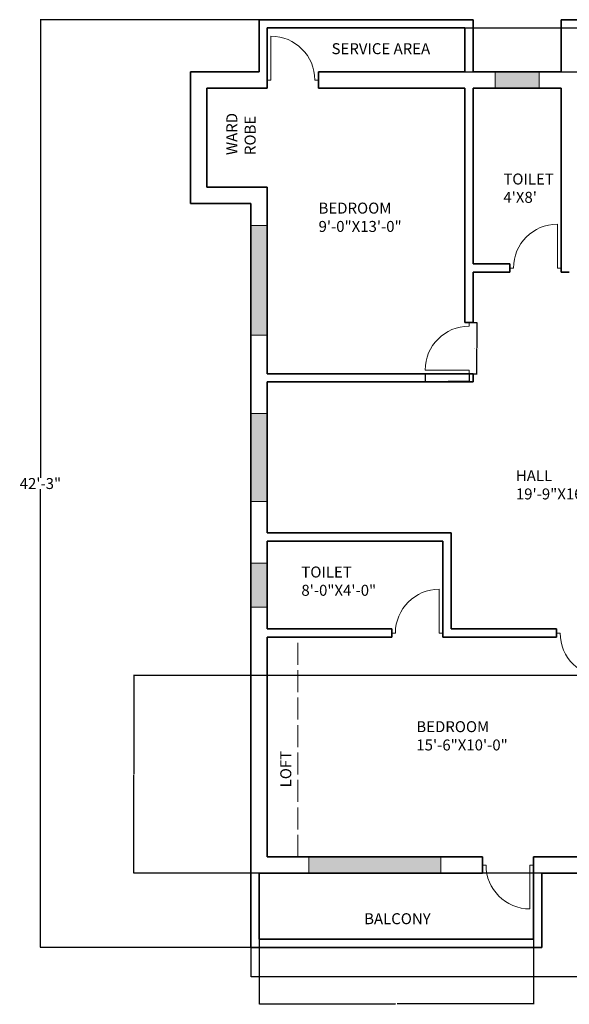
# Model space of a CAD drawing. Units: inches. Extents: x -89 to 565, y -517 to 71.
# Tile 1 of 3: x -89 to 211, y -499 to 39. Entities that reach past the tile are written whole.
import ezdxf

# ---------------------------------------------------------------- set-up
doc = ezdxf.new("R2010")
doc.units = ezdxf.units.IN
doc.header["$MEASUREMENT"] = 0
doc.linetypes.add('ACAD_ISO02W100', pattern=[15, 12, -3])
for name, color, linetype, lineweight in [('A-ANNO-DIMS', 2, 'Continuous', 18), ('A-AREA-IDEN', 7, 'Continuous', 18), ('A-DOOR', 4, 'Continuous', 18), ('A-FLOR-OVHD', 8, 'ACAD_ISO02W100', 18), ('A-GLAZ', 3, 'Continuous', 18), ('A-GLAZ-PATT', 9, 'Continuous', 13), ('A-WALL', 7, 'Continuous', 35)]:
    doc.layers.add(name, color=color, linetype=linetype, lineweight=lineweight)
doc.styles.get("Standard").update_dxf_attribs({"font": 'arial.ttf'})
doc.dimstyles.get("Standard").update_dxf_attribs({"dimtxt": 0.18, "dimasz": 0.18, "dimexe": 0.18, "dimexo": 0.0625, "dimgap": 0.09, "dimtad": 0, "dimtih": 1, "dimtoh": 1, "dimdec": 0, "dimzin": 0, "dimdsep": 46, "dimlunit": 3, "dimtxsty": 'Standard', "dimcen": 0.09, "dimadec": 0, "dimazin": 0, "dimtfac": 1, "dimtdec": 0, "dimtofl": 0, "dimtmove": 0, "dimatfit": 3, "dimfxl": 1, "dimtolj": 1, "dimtzin": 0, "dimarcsym": 0})

# ---------------------------------------------------------------- blocks, each defined once
blk = doc.blocks.new('*D2')
at = {"layer": 'A-ANNO-DIMS', "color": 0, "lineweight": -2, "transparency": 16777216}
for p, q in [((37.09, -467.65), (37.09, -483.62)), ((533.59, -467.65), (533.59, -483.62)), ((37.27, -483.44), (274.83, -483.44)), ((533.41, -483.44), (295.86, -483.44))]:
    blk.add_line(p, q, dxfattribs=at)
at = {"layer": 'A-ANNO-DIMS', "color": 0, "transparency": 16777216}
for points in [[(37.27, -483.41), (37.27, -483.47), (37.09, -483.44)], [(533.41, -483.41), (533.41, -483.47), (533.59, -483.44)]]:
    blk.add_solid(points, dxfattribs=at)
at = {"layer": 'Defpoints', "color": 0, "transparency": 16777216}
for p in [(37.09, -467.59), (533.59, -467.59), (533.59, -483.44)]:
    blk.add_point(p, dxfattribs=at)
at = {"layer": 'A-ANNO-DIMS', "color": 0, "transparency": 16777216, "insert": (285.34, -483.44), "char_height": 6, "attachment_point": 5}
blk.add_mtext('\\A1;41\'-5"', dxfattribs=at)
blk = doc.blocks.new('*D3')
at = {"layer": 'A-ANNO-DIMS', "color": 0, "lineweight": -2, "transparency": 16777216}
for p, q in [((41.53, 39.41), (-78.02, 39.41)), ((-77.84, 39.23), (-77.84, -210.93)), ((-77.84, -467.41), (-77.84, -217.24)), ((37.03, -467.59), (-78.02, -467.59))]:
    blk.add_line(p, q, dxfattribs=at)
at = {"layer": 'A-ANNO-DIMS', "color": 0, "transparency": 16777216}
for points in [[(-77.87, 39.23), (-77.81, 39.23), (-77.84, 39.41)], [(-77.87, -467.41), (-77.81, -467.41), (-77.84, -467.59)]]:
    blk.add_solid(points, dxfattribs=at)
at = {"layer": 'Defpoints', "color": 0, "transparency": 16777216}
for p in [(-77.84, 39.41), (41.59, 39.41), (37.09, -467.59)]:
    blk.add_point(p, dxfattribs=at)
at = {"layer": 'A-ANNO-DIMS', "color": 0, "transparency": 16777216, "insert": (-77.84, -214.09), "char_height": 6, "attachment_point": 5}
blk.add_mtext('\\A1;42\'-3"', dxfattribs=at)
blk = doc.blocks.new('DOOR-SWING-24IN')
for p, q in [((0, 0), (0, 24)), ((-24, 0), (-26, 0)), ((2, 0), (0, 0))]:
    blk.add_line(p, q)
blk.add_arc((0, 0), 24, 90, 180)
blk = doc.blocks.new('*D10')
at = {"layer": 'A-ANNO-DIMS', "color": 0, "lineweight": -2, "transparency": 16777216}
for p, q in [((156.41, -126.09), (160.72, -126.09)), ((160.54, -126.27), (160.54, -139.9)), ((160.54, -153.91), (160.54, -140.27)), ((156.41, -154.09), (160.72, -154.09))]:
    blk.add_line(p, q, dxfattribs=at)
at = {"layer": 'A-ANNO-DIMS', "color": 0, "transparency": 16777216}
for points in [[(160.51, -126.27), (160.57, -126.27), (160.54, -126.09)], [(160.51, -153.91), (160.57, -153.91), (160.54, -154.09)]]:
    blk.add_solid(points, dxfattribs=at)
at = {"layer": 'Defpoints', "color": 0, "transparency": 16777216}
for p in [(156.34, -126.09), (156.34, -154.09), (160.54, -154.09)]:
    blk.add_point(p, dxfattribs=at)
at = {"layer": 'A-ANNO-DIMS', "color": 0, "transparency": 16777216, "insert": (160.54, -140.09), "char_height": 0.18, "attachment_point": 5}
blk.add_mtext('\\A1;PASSAGE DOOR 2\'-4" TYP.', dxfattribs=at)
blk = doc.blocks.new('*D11')
at = {"layer": 'A-ANNO-DIMS', "color": 0, "lineweight": -2, "transparency": 16777216}
for p, q in [((132.34, -154.15), (132.34, -158.47)), ((156.34, -154.15), (156.34, -158.47)), ((132.52, -158.29), (143.7, -158.29)), ((156.16, -158.29), (144.98, -158.29))]:
    blk.add_line(p, q, dxfattribs=at)
at = {"layer": 'A-ANNO-DIMS', "color": 0, "transparency": 16777216}
for points in [[(132.52, -158.26), (132.52, -158.32), (132.34, -158.29)], [(156.16, -158.26), (156.16, -158.32), (156.34, -158.29)]]:
    blk.add_solid(points, dxfattribs=at)
at = {"layer": 'Defpoints', "color": 0, "transparency": 16777216}
for p in [(132.34, -154.09), (156.34, -154.09), (132.34, -158.29)]:
    blk.add_point(p, dxfattribs=at)
at = {"layer": 'A-ANNO-DIMS', "color": 0, "transparency": 16777216, "insert": (144.34, -158.29), "char_height": 0.18, "attachment_point": 5}
blk.add_mtext('\\A1;2\'-0" TYP.', dxfattribs=at)
blk = doc.blocks.new('*D27')
at = {"layer": 'A-ANNO-DIMS', "color": 0, "lineweight": -2, "transparency": 16777216}
for p, q in [((241.03, -319.09), (-27.04, -319.09)), ((-26.86, -319.27), (-26.86, -372.9)), ((-26.86, -426.91), (-26.86, -373.27)), ((241.03, -427.09), (-27.04, -427.09))]:
    blk.add_line(p, q, dxfattribs=at)
at = {"layer": 'A-ANNO-DIMS', "color": 0, "transparency": 16777216}
for points in [[(-26.89, -319.27), (-26.83, -319.27), (-26.86, -319.09)], [(-26.89, -426.91), (-26.83, -426.91), (-26.86, -427.09)]]:
    blk.add_solid(points, dxfattribs=at)
at = {"layer": 'Defpoints', "color": 0, "transparency": 16777216}
for p in [(241.09, -319.09), (-26.86, -427.09), (241.09, -427.09)]:
    blk.add_point(p, dxfattribs=at)
at = {"layer": 'A-ANNO-DIMS', "color": 0, "transparency": 16777216, "insert": (-26.86, -373.09), "char_height": 0.18, "attachment_point": 5}
blk.add_mtext('\\A1;9\'-0"', dxfattribs=at)
blk = doc.blocks.new('*D30')
at = {"layer": 'A-ANNO-DIMS', "color": 0, "lineweight": -2, "transparency": 16777216}
for p, q in [((41.59, -463.15), (41.59, -498.72)), ((191.59, -463.15), (191.59, -498.72)), ((41.77, -498.54), (116.2, -498.54)), ((191.41, -498.54), (116.98, -498.54))]:
    blk.add_line(p, q, dxfattribs=at)
at = {"layer": 'A-ANNO-DIMS', "color": 0, "transparency": 16777216}
for points in [[(41.77, -498.51), (41.77, -498.57), (41.59, -498.54)], [(191.41, -498.51), (191.41, -498.57), (191.59, -498.54)]]:
    blk.add_solid(points, dxfattribs=at)
at = {"layer": 'Defpoints', "color": 0, "transparency": 16777216}
for p in [(41.59, -463.09), (191.59, -463.09), (191.59, -498.54)]:
    blk.add_point(p, dxfattribs=at)
at = {"layer": 'A-ANNO-DIMS', "color": 0, "transparency": 16777216, "insert": (116.59, -498.54), "char_height": 0.18, "attachment_point": 5}
blk.add_mtext('\\A1;12\'-6"', dxfattribs=at)
blk = doc.blocks.new('*D33')
at = {"layer": 'A-ANNO-DIMS', "color": 0, "lineweight": -2, "transparency": 16777216}
for p, q in [((154.16, 34.91), (564.72, 34.91)), ((564.54, 34.73), (564.54, 23.1)), ((564.54, 11.09), (564.54, 22.73)), ((154.16, 10.91), (564.72, 10.91))]:
    blk.add_line(p, q, dxfattribs=at)
at = {"layer": 'A-ANNO-DIMS', "color": 0, "transparency": 16777216}
for points in [[(564.51, 34.73), (564.57, 34.73), (564.54, 34.91)], [(564.51, 11.09), (564.57, 11.09), (564.54, 10.91)]]:
    blk.add_solid(points, dxfattribs=at)
at = {"layer": 'Defpoints', "color": 0, "transparency": 16777216}
for p in [(154.09, 34.91), (564.54, 34.91), (154.09, 10.91)]:
    blk.add_point(p, dxfattribs=at)
at = {"layer": 'A-ANNO-DIMS', "color": 0, "transparency": 16777216, "insert": (564.54, 22.91), "char_height": 0.18, "attachment_point": 5}
blk.add_mtext('\\A1;2\'-0"', dxfattribs=at)

msp = doc.modelspace()

# ---------------------------------------------------------------- hatches: boundary and pattern name
at = {"layer": 'A-GLAZ-PATT'}
h = msp.add_hatch(dxfattribs=at)
h.set_pattern_fill('GOST_WOOD', color=256)
h.set_pattern_definition([(90, (0, 0), (6, -4e-16), [10, -2]), (90, (2, -2), (6, -4e-16), [6, -1.5, 3, -1.5]), (90, (4, -5), (6, -4e-16), [10, -2])])
h.paths.add_polyline_path([(46.09, -73.09), (41.59, -73.09), (37.09, -73.09), (37.09, -133.09), (41.59, -133.09), (46.09, -133.09)])
h.paths.add_polyline_path([(46.09, -175.84), (41.59, -175.84), (37.09, -175.84), (37.09, -223.84), (41.59, -223.84), (46.09, -223.84)])
h.paths.add_polyline_path([(46.09, -257.59), (41.59, -257.59), (37.09, -257.59), (37.09, -281.59), (41.59, -281.59), (46.09, -281.59)])
h.paths.add_polyline_path([(140.84, -418.09), (68.84, -418.09), (68.84, -422.59), (68.84, -427.09), (140.84, -427.09), (140.84, -422.59)])
h.paths.add_polyline_path([(501.84, -418.09), (429.84, -418.09), (429.84, -422.59), (429.84, -427.09), (501.84, -427.09), (501.84, -422.59)])
h.paths.add_polyline_path([(533.59, -322.09), (529.09, -322.09), (524.59, -322.09), (524.59, -394.09), (529.09, -394.09), (533.59, -394.09)])
h.paths.add_polyline_path([(533.59, -257.59), (529.09, -257.59), (524.59, -257.59), (524.59, -281.59), (529.09, -281.59), (533.59, -281.59)])
h.paths.add_polyline_path([(533.59, -205.09), (529.09, -205.09), (524.59, -205.09), (524.59, -229.09), (529.09, -229.09), (533.59, -229.09)])
h.paths.add_polyline_path([(533.59, -148.09), (529.09, -148.09), (524.59, -148.09), (524.59, -172.09), (529.09, -172.09), (533.59, -172.09)])
h.paths.add_polyline_path([(533.59, -26.59), (529.09, -26.59), (524.59, -26.59), (524.59, -98.59), (529.09, -98.59), (533.59, -98.59)])
h.paths.add_polyline_path([(421.09, 10.91), (365.78, 10.91), (365.78, 1.91), (421.09, 1.91)])
h.paths.add_polyline_path([(194.59, 10.91), (170.59, 10.91), (170.59, 1.91), (194.59, 1.91)])

# ---------------------------------------------------------------- linework, layer by layer
at = {"layer": 'A-FLOR-OVHD'}
msp.add_line((62.75, -418.09), (62.75, -298.09), dxfattribs=at)
at = {"layer": 'A-GLAZ'}
for p, q in [((170.59, 1.91), (170.59, 10.91)), ((194.59, 1.91), (194.59, 10.91)), ((41.59, -73.09), (37.09, -73.09)), ((41.59, -73.09), (46.09, -73.09)), ((41.59, -133.09), (37.09, -133.09)), ((41.59, -133.09), (46.09, -133.09)), ((41.59, -175.84), (37.09, -175.84)), ((41.59, -175.84), (46.09, -175.84)), ((41.59, -223.84), (37.09, -223.84)), ((41.59, -223.84), (46.09, -223.84)), ((46.09, -223.84), (46.09, -223.84)), ((41.59, -257.59), (37.09, -257.59)), ((41.59, -257.59), (46.09, -257.59)), ((41.59, -281.59), (37.09, -281.59)), ((41.59, -281.59), (46.09, -281.59)), ((68.84, -422.59), (68.84, -418.09)), ((140.84, -422.59), (140.84, -418.09)), ((68.84, -422.59), (68.84, -427.09)), ((140.84, -422.59), (140.84, -427.09))]:
    msp.add_line(p, q, dxfattribs=at)
at = {"layer": 'A-WALL'}
for p, q in [((41.59, 34.91), (41.59, 39.41)), ((41.59, 39.41), (46.09, 39.41)), ((46.09, 39.41), (128.89, 39.41)), ((128.89, 39.41), (158.59, 39.41)), ((158.59, 10.91), (158.59, 39.41)), ((206.59, 10.91), (206.59, 39.41)), ((206.59, 39.41), (533.59, 39.41)), ((41.59, 10.91), (41.59, 34.91)), ((46.09, 10.91), (46.09, 34.91)), ((46.09, 34.91), (128.89, 34.91)), ((154.09, 34.91), (128.89, 34.91)), ((154.09, 10.91), (154.09, 34.91)), ((4.09, 1.91), (4.09, 10.91)), ((4.09, 10.91), (13.09, 10.91)), ((37.09, 10.91), (13.09, 10.91)), ((37.09, 10.91), (41.59, 10.91)), ((46.09, 1.91), (46.09, 10.91)), ((74.09, 6.41), (74.09, 10.91)), ((74.09, 10.91), (154.09, 10.91)), ((158.59, 10.91), (206.59, 10.91)), ((74.09, 6.41), (74.09, 1.91)), ((4.09, 1.91), (4.09, -34.09)), ((37.09, 1.91), (13.09, 1.91)), ((13.09, 1.91), (13.09, -34.09)), ((37.09, 1.91), (46.09, 1.91)), ((74.09, 1.91), (154.09, 1.91)), ((154.09, 1.91), (154.09, -126.09)), ((158.59, 1.91), (158.59, -94.09)), ((158.59, 1.91), (206.59, 1.91)), ((206.59, 1.91), (206.59, -98.59)), ((4.09, -34.09), (4.09, -52.09)), ((13.09, -34.09), (13.09, -52.09)), ((4.09, -52.09), (4.09, -61.09)), ((13.09, -52.09), (14.95, -52.09)), ((46.09, -52.09), (14.95, -52.09)), ((46.09, -52.09), (46.09, -154.09)), ((4.09, -61.09), (14.95, -61.09)), ((37.09, -61.09), (14.95, -61.09)), ((37.09, -61.09), (37.09, -467.59)), ((158.59, -94.09), (178.59, -94.09)), ((178.59, -96.34), (178.59, -94.09)), ((178.59, -96.34), (178.59, -98.59)), ((158.59, -98.59), (178.59, -98.59)), ((158.59, -98.59), (158.59, -126.09)), ((206.59, -98.59), (211.09, -98.59)), ((156.34, -126.09), (154.09, -126.09)), ((156.34, -126.09), (158.59, -126.09)), ((46.09, -154.09), (158.59, -154.09)), ((158.59, -154.09), (158.59, -158.59)), ((46.09, -158.59), (158.59, -158.59)), ((46.09, -158.59), (46.09, -241.09)), ((46.09, -241.09), (146.59, -241.09)), ((146.59, -241.09), (146.59, -293.59)), ((46.09, -245.59), (142.09, -245.59)), ((46.09, -245.59), (46.09, -293.59)), ((142.09, -245.59), (142.09, -298.09)), ((46.09, -293.59), (114.09, -293.59)), ((46.09, -293.59), (114.09, -293.59)), ((114.09, -295.84), (114.09, -293.59)), ((114.09, -295.84), (114.09, -298.09)), ((146.59, -293.59), (204.09, -293.59)), ((204.09, -295.84), (204.09, -293.59)), ((204.09, -295.84), (204.09, -298.09)), ((46.09, -298.09), (114.09, -298.09)), ((46.09, -298.09), (46.09, -418.09)), ((142.09, -298.09), (204.09, -298.09)), ((46.09, -418.09), (163.59, -418.09)), ((163.59, -422.59), (163.59, -418.09)), ((191.59, -418.09), (191.59, -463.09)), ((191.59, -418.09), (232.09, -418.09)), ((163.59, -422.59), (163.59, -427.09)), ((46.09, -427.09), (41.59, -427.09)), ((41.59, -427.09), (41.59, -463.09)), ((46.09, -427.09), (163.59, -427.09)), ((196.09, -427.09), (196.09, -467.59)), ((196.09, -427.09), (232.09, -427.09)), ((37.09, -467.59), (196.09, -467.59)), ((41.59, -463.09), (191.59, -463.09))]:
    msp.add_line(p, q, dxfattribs=at)

# ---------------------------------------------------------------- block references
at = {"layer": 'A-DOOR', "extrusion": (0, 0, -1), "zscale": -1}
msp.add_blockref('DOOR-SWING-24IN', (-48.09, 6.41), dxfattribs=at)
at = {"layer": 'A-DOOR'}
for p in [(204.59, -96.34), (140.09, -295.84)]:
    msp.add_blockref('DOOR-SWING-24IN', p, dxfattribs=at)
at = {"layer": 'A-DOOR', "extrusion": (0, 0, -1), "zscale": -1}
for p, rotation in [((-156.34, -152.09), 270), ((-230.09, -295.84), 180), ((-189.59, -422.59), 180)]:
    msp.add_blockref('DOOR-SWING-24IN', p, dxfattribs=dict(at, rotation=rotation))

# ---------------------------------------------------------------- texts
at = {"layer": 'A-AREA-IDEN', "char_height": 6, "attachment_point": 1}
for s, insert in [('SERVICE AREA', (81.22, 26.57)), ("TOILET\\P4'X8'", (175.08, -44.67)), ('BEDROOM\\P9\'-0"X13\'-0"', (74.11, -60.57)), ('HALL\\P19\'-9"X16\'-3"', (181.9, -206.79)), ('TOILET\\P8\'-0"X4\'-0"', (64.72, -259.45)), ('BEDROOM\\P15\'-6"X10\'-0"', (127.53, -343.98)), ('BALCONY', (99.01, -448.93))]:
    msp.add_mtext(s, dxfattribs=dict(at, insert=insert))
at = {"layer": 'A-AREA-IDEN', "char_height": 6, "attachment_point": 1, "rotation": 90}
for s, insert in [('WARD\\PROBE', (23.74, -34.57)), ('LOFT', (53.22, -380.14))]:
    msp.add_mtext(s, dxfattribs=dict(at, insert=insert))

# ---------------------------------------------------------------- dimensions: what is measured, and where the dimension line sits
at = {"layer": 'A-ANNO-DIMS'}
for base, p1, p2, override, picture, middle in [((-77.84, 39.41), (37.09, -467.59), (41.59, 39.41), {"dimtxt": 6, "dimclrd": 0, "dimclre": 0, "dimclrt": 0}, '*D3', (-77.84, -214.09)), ((564.54, 34.91), (154.09, 10.91), (154.09, 34.91), {"dimdec": 1, "dimlfac": 1, "dimrnd": 0, "dimzin": 1, "dimdsep": 46, "dimlunit": 4, "dimfrac": 2}, '*D33', (564.54, 22.91)), ((-26.86, -427.09), (241.09, -319.09), (241.09, -427.09), {"dimdec": 1, "dimlfac": 1, "dimrnd": 0, "dimzin": 1, "dimdsep": 46, "dimlunit": 4, "dimfrac": 2}, '*D27', (-26.86, -373.09))]:
    dim = msp.add_linear_dim(base=base, p1=p1, p2=p2, angle=90, dimstyle='Standard', override=override, dxfattribs=at)
    dim.commit()
    dim.dimension.update_dxf_attribs({"geometry": picture, "text_midpoint": middle})
for base, p1, p2, angle, text, picture, middle in [((160.54, -154.09), (156.34, -126.09), (156.34, -154.09), 270, 'PASSAGE DOOR <> TYP.', '*D10', (160.54, -140.09)), ((132.34, -158.29), (156.34, -154.09), (132.34, -154.09), 180, '<> TYP.', '*D11', (144.34, -158.29))]:
    dim = msp.add_linear_dim(base=base, p1=p1, p2=p2, angle=angle, text=text, dimstyle='Standard', override={"dimdec": 1, "dimlfac": 1, "dimrnd": 0, "dimzin": 1, "dimdsep": 46, "dimlunit": 4, "dimfrac": 2}, dxfattribs=at)
    dim.commit()
    dim.dimension.update_dxf_attribs({"geometry": picture, "text_midpoint": middle})
for base, p1, p2, override, picture, middle in [((533.59381792, -483.44106033), (37.09381792, -467.58551125), (533.59381792, -467.58551125), {"dimtxt": 6, "dimclrd": 0, "dimclre": 0, "dimclrt": 0}, '*D2', (285.34381792, -483.44106033)), ((191.59, -498.54), (41.59, -463.09), (191.59, -463.09), {"dimdec": 1, "dimlfac": 1, "dimrnd": 0, "dimzin": 1, "dimdsep": 46, "dimlunit": 4, "dimfrac": 2}, '*D30', (116.59, -498.54))]:
    dim = msp.add_linear_dim(base=base, p1=p1, p2=p2, dimstyle='Standard', override=override, dxfattribs=at)
    dim.commit()
    dim.dimension.update_dxf_attribs({"geometry": picture, "text_midpoint": middle})

doc.saveas('drawing.dxf')
